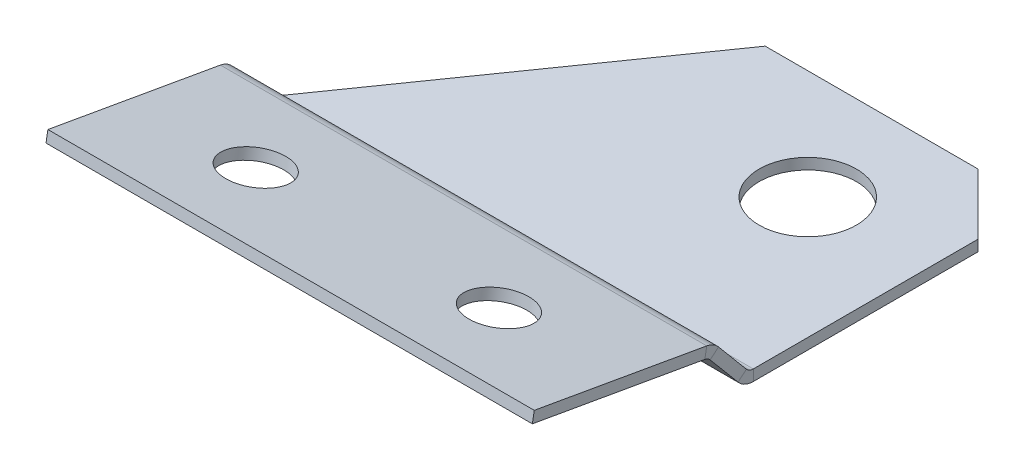
ISO-10303-21;
HEADER;
FILE_DESCRIPTION(('STEP AP214'),'2;1');
FILE_NAME('part.step','',(''),(''),'','','');
FILE_SCHEMA(('AUTOMOTIVE_DESIGN { 1 0 10303 214 1 1 1 1 }'));
ENDSEC;
DATA;
#1=APPLICATION_CONTEXT('core data for automotive mechanical design processes');
#2=APPLICATION_PROTOCOL_DEFINITION('international standard','automotive_design',2000,#1);
#3=PRODUCT_CONTEXT('',#1,'mechanical');
#4=PRODUCT('Part','Part','',(#3));
#5=PRODUCT_RELATED_PRODUCT_CATEGORY('part','',(#4));
#6=PRODUCT_DEFINITION_FORMATION('','',#4);
#7=PRODUCT_DEFINITION_CONTEXT('part definition',#1,'design');
#8=PRODUCT_DEFINITION('design','',#6,#7);
#9=PRODUCT_DEFINITION_SHAPE('','',#8);
#10=(LENGTH_UNIT() NAMED_UNIT(*) SI_UNIT(.MILLI.,.METRE.));
#11=(NAMED_UNIT(*) PLANE_ANGLE_UNIT() SI_UNIT($,.RADIAN.));
#12=(NAMED_UNIT(*) SI_UNIT($,.STERADIAN.) SOLID_ANGLE_UNIT());
#13=UNCERTAINTY_MEASURE_WITH_UNIT(LENGTH_MEASURE(1.E-05),#10,'distance_accuracy_value','');
#14=(GEOMETRIC_REPRESENTATION_CONTEXT(3) GLOBAL_UNCERTAINTY_ASSIGNED_CONTEXT((#13)) GLOBAL_UNIT_ASSIGNED_CONTEXT((#10,
#11,#12)) REPRESENTATION_CONTEXT('',''));
#15=CARTESIAN_POINT('',(0.,0.,0.));
#16=DIRECTION('',(0.,0.,1.));
#17=DIRECTION('',(1.,0.,0.));
#18=AXIS2_PLACEMENT_3D('',#15,#16,#17);
#19=CARTESIAN_POINT('',(-7.56166635581271,4.19626665871385,33.5211914025943));
#20=DIRECTION('',(-1.,0.,0.));
#21=DIRECTION('',(0.,0.,1.));
#22=AXIS2_PLACEMENT_3D('',#19,#20,#21);
#23=PLANE('',#22);
#24=DIRECTION('',(0.,0.766044443118975,0.642787609686544));
#25=VECTOR('',#24,1.);
#26=CARTESIAN_POINT('',(-7.56166635581271,4.19626665871385,33.5211914025943));
#27=LINE('',#26,#25);
#28=CARTESIAN_POINT('',(-7.56166635581271,0.184613797987,30.1550149667471));
#29=VERTEX_POINT('',#28);
#30=CARTESIAN_POINT('',(-7.56166635581271,2.91831154664444,32.4488597393957));
#31=VERTEX_POINT('',#30);
#32=EDGE_CURVE('E254',#29,#31,#27,.T.);
#33=ORIENTED_EDGE('',*,*,#32,.T.);
#34=DIRECTION('',(0.,0.642787609686544,-0.766044443118974));
#35=VECTOR('',#34,1.);
#36=CARTESIAN_POINT('',(-7.56166635581271,2.91831154664444,32.4488597393957));
#37=LINE('',#36,#35);
#38=CARTESIAN_POINT('',(-7.56166635581271,3.49682039536233,31.7594197405887));
#39=VERTEX_POINT('',#38);
#40=EDGE_CURVE('E241',#31,#39,#37,.T.);
#41=ORIENTED_EDGE('',*,*,#40,.T.);
#42=DIRECTION('',(0.,-0.766044443118975,-0.642787609686544));
#43=VECTOR('',#42,1.);
#44=CARTESIAN_POINT('',(-7.56166635581271,-14.7721682915287,16.4299180714363));
#45=LINE('',#44,#43);
#46=CARTESIAN_POINT('',(-7.56166635581271,0.76312264670489,29.46557496794));
#47=VERTEX_POINT('',#46);
#48=EDGE_CURVE('E259',#47,#39,#45,.F.);
#49=ORIENTED_EDGE('',*,*,#48,.F.);
#50=DIRECTION('',(0.,-0.642787609686544,0.766044443118974));
#51=VECTOR('',#50,1.);
#52=CARTESIAN_POINT('',(-7.56166635581271,0.184613797987001,30.1550149667471));
#53=LINE('',#52,#51);
#54=EDGE_CURVE('E247',#47,#29,#53,.T.);
#55=ORIENTED_EDGE('',*,*,#54,.T.);
#56=EDGE_LOOP('',(#33,#41,#49,#55));
#57=FACE_BOUND('',#56,.T.);
#58=ADVANCED_FACE('F81',(#57),#23,.T.);
#59=CARTESIAN_POINT('',(0.,-15.3506771402466,17.1193580702434));
#60=DIRECTION('',(0.,-0.642787609686544,0.766044443118975));
#61=DIRECTION('',(0.,-0.766044443118975,-0.642787609686544));
#62=AXIS2_PLACEMENT_3D('',#59,#60,#61);
#63=PLANE('',#62);
#64=DIRECTION('',(0.,-0.766044443118975,-0.642787609686544));
#65=VECTOR('',#64,1.);
#66=CARTESIAN_POINT('',(32.4383336441873,-0.0785088487178904,29.9342288509426));
#67=LINE('',#66,#65);
#68=CARTESIAN_POINT('',(32.4383336441873,2.91831154664445,32.4488597393957));
#69=VERTEX_POINT('',#68);
#70=CARTESIAN_POINT('',(32.4383336441873,0.184613797987,30.1550149667471));
#71=VERTEX_POINT('',#70);
#72=EDGE_CURVE('E249',#69,#71,#67,.T.);
#73=ORIENTED_EDGE('',*,*,#72,.F.);
#74=DIRECTION('',(-1.,0.,0.));
#75=VECTOR('',#74,1.);
#76=CARTESIAN_POINT('',(-7.56166635581271,2.91831154664444,32.4488597393957));
#77=LINE('',#76,#75);
#78=EDGE_CURVE('E107',#31,#69,#77,.F.);
#79=ORIENTED_EDGE('',*,*,#78,.F.);
#80=ORIENTED_EDGE('',*,*,#32,.F.);
#81=DIRECTION('',(1.,0.,0.));
#82=VECTOR('',#81,1.);
#83=CARTESIAN_POINT('',(0.,0.184613797986996,30.1550149667471));
#84=LINE('',#83,#82);
#85=EDGE_CURVE('E256',#29,#71,#84,.T.);
#86=ORIENTED_EDGE('',*,*,#85,.T.);
#87=EDGE_LOOP('',(#73,#79,#80,#86));
#88=FACE_BOUND('',#87,.T.);
#89=ADVANCED_FACE('F321',(#88),#63,.T.);
#90=CARTESIAN_POINT('',(0.,-14.7721682915287,16.4299180714363));
#91=DIRECTION('',(0.,-0.642787609686544,0.766044443118975));
#92=DIRECTION('',(0.,-0.766044443118975,-0.642787609686544));
#93=AXIS2_PLACEMENT_3D('',#90,#91,#92);
#94=PLANE('',#93);
#95=DIRECTION('',(-1.,0.,0.));
#96=VECTOR('',#95,1.);
#97=CARTESIAN_POINT('',(-7.56166635581271,3.49682039536233,31.7594197405887));
#98=LINE('',#97,#96);
#99=CARTESIAN_POINT('',(32.4383336441873,3.49682039536233,31.7594197405887));
#100=VERTEX_POINT('',#99);
#101=EDGE_CURVE('E188',#39,#100,#98,.F.);
#102=ORIENTED_EDGE('',*,*,#101,.T.);
#103=DIRECTION('',(0.,0.766044443118975,0.642787609686544));
#104=VECTOR('',#103,1.);
#105=CARTESIAN_POINT('',(32.4383336441873,-14.7721682915287,16.4299180714363));
#106=LINE('',#105,#104);
#107=CARTESIAN_POINT('',(32.4383336441873,0.76312264670489,29.46557496794));
#108=VERTEX_POINT('',#107);
#109=EDGE_CURVE('E253',#100,#108,#106,.F.);
#110=ORIENTED_EDGE('',*,*,#109,.T.);
#111=DIRECTION('',(-1.,0.,0.));
#112=VECTOR('',#111,1.);
#113=CARTESIAN_POINT('',(-7.56166635581271,0.763122646704892,29.46557496794));
#114=LINE('',#113,#112);
#115=EDGE_CURVE('E268',#47,#108,#114,.F.);
#116=ORIENTED_EDGE('',*,*,#115,.F.);
#117=ORIENTED_EDGE('',*,*,#48,.T.);
#118=EDGE_LOOP('',(#102,#110,#116,#117));
#119=FACE_BOUND('',#118,.T.);
#120=ADVANCED_FACE('F330',(#119),#94,.F.);
#121=CARTESIAN_POINT('',(32.4383336441873,0.5,0.));
#122=DIRECTION('',(-1.,0.,0.));
#123=DIRECTION('',(0.,0.,1.));
#124=AXIS2_PLACEMENT_3D('',#121,#122,#123);
#125=PLANE('',#124);
#126=DIRECTION('',(0.,0.,1.));
#127=VECTOR('',#126,1.);
#128=CARTESIAN_POINT('',(32.4383336441873,0.5,0.));
#129=LINE('',#128,#127);
#130=CARTESIAN_POINT('',(32.4383336441873,0.5,10.4196554125346));
#131=VERTEX_POINT('',#130);
#132=CARTESIAN_POINT('',(32.4383336441873,0.5,28.9013066311386));
#133=VERTEX_POINT('',#132);
#134=EDGE_CURVE('E379',#131,#133,#129,.T.);
#135=ORIENTED_EDGE('',*,*,#134,.T.);
#136=DIRECTION('',(0.,-1.,0.));
#137=VECTOR('',#136,1.);
#138=CARTESIAN_POINT('',(32.4383336441873,0.499999999999996,28.9013066311386));
#139=LINE('',#138,#137);
#140=CARTESIAN_POINT('',(32.4383336441873,-0.400000000000005,28.9013066311386));
#141=VERTEX_POINT('',#140);
#142=EDGE_CURVE('E282',#133,#141,#139,.T.);
#143=ORIENTED_EDGE('',*,*,#142,.T.);
#144=DIRECTION('',(0.,0.,1.));
#145=VECTOR('',#144,1.);
#146=CARTESIAN_POINT('',(32.4383336441873,-0.4,0.));
#147=LINE('',#146,#145);
#148=CARTESIAN_POINT('',(32.4383336441873,-0.4,10.4196554125346));
#149=VERTEX_POINT('',#148);
#150=EDGE_CURVE('E366',#149,#141,#147,.T.);
#151=ORIENTED_EDGE('',*,*,#150,.F.);
#152=DIRECTION('',(0.,1.,0.));
#153=VECTOR('',#152,1.);
#154=CARTESIAN_POINT('',(32.4383336441873,0.5,10.4196554125346));
#155=LINE('',#154,#153);
#156=EDGE_CURVE('E13',#149,#131,#155,.T.);
#157=ORIENTED_EDGE('',*,*,#156,.T.);
#158=EDGE_LOOP('',(#135,#143,#151,#157));
#159=FACE_BOUND('',#158,.T.);
#160=ADVANCED_FACE('F420',(#159),#125,.F.);
#161=CARTESIAN_POINT('',(9.21616941809498,0.5,6.45131859266648));
#162=DIRECTION('',(-0.81923192051904,0.,-0.573462344363328));
#163=DIRECTION('',(-0.573462344363328,0.,0.81923192051904));
#164=AXIS2_PLACEMENT_3D('',#161,#162,#163);
#165=PLANE('',#164);
#166=DIRECTION('',(-0.573462344363328,0.,0.81923192051904));
#167=VECTOR('',#166,1.);
#168=CARTESIAN_POINT('',(9.21616941809498,-0.4,6.45131859266648));
#169=LINE('',#168,#167);
#170=CARTESIAN_POINT('',(9.93833364418729,-0.4,5.41965541253461));
#171=VERTEX_POINT('',#170);
#172=CARTESIAN_POINT('',(-6.49882220883548,-0.4,28.9013066311386));
#173=VERTEX_POINT('',#172);
#174=EDGE_CURVE('E361',#171,#173,#169,.T.);
#175=ORIENTED_EDGE('',*,*,#174,.T.);
#176=DIRECTION('',(0.,-1.,0.));
#177=VECTOR('',#176,1.);
#178=CARTESIAN_POINT('',(-6.49882220883548,0.499999999999996,28.9013066311386));
#179=LINE('',#178,#177);
#180=CARTESIAN_POINT('',(-6.49882220883548,0.5,28.9013066311386));
#181=VERTEX_POINT('',#180);
#182=EDGE_CURVE('E281',#181,#173,#179,.T.);
#183=ORIENTED_EDGE('',*,*,#182,.F.);
#184=DIRECTION('',(-0.573462344363328,0.,0.81923192051904));
#185=VECTOR('',#184,1.);
#186=CARTESIAN_POINT('',(9.21616941809498,0.5,6.45131859266648));
#187=LINE('',#186,#185);
#188=CARTESIAN_POINT('',(9.93833364418729,0.5,5.41965541253461));
#189=VERTEX_POINT('',#188);
#190=EDGE_CURVE('E384',#189,#181,#187,.T.);
#191=ORIENTED_EDGE('',*,*,#190,.F.);
#192=DIRECTION('',(0.,1.,0.));
#193=VECTOR('',#192,1.);
#194=CARTESIAN_POINT('',(9.93833364418729,0.5,5.41965541253461));
#195=LINE('',#194,#193);
#196=EDGE_CURVE('E360',#171,#189,#195,.T.);
#197=ORIENTED_EDGE('',*,*,#196,.F.);
#198=EDGE_LOOP('',(#175,#183,#191,#197));
#199=FACE_BOUND('',#198,.T.);
#200=ADVANCED_FACE('F89',(#199),#165,.T.);
#201=CARTESIAN_POINT('',(0.,0.5,0.));
#202=DIRECTION('',(0.,1.,0.));
#203=DIRECTION('',(0.,0.,1.));
#204=AXIS2_PLACEMENT_3D('',#201,#202,#203);
#205=PLANE('',#204);
#206=CARTESIAN_POINT('',(22.4383336441873,0.5,14.4196554125346));
#207=DIRECTION('',(0.,1.,0.));
#208=DIRECTION('',(0.,0.,1.));
#209=AXIS2_PLACEMENT_3D('',#206,#207,#208);
#210=CIRCLE('',#209,4.);
#211=CARTESIAN_POINT('',(22.4383336441873,0.5,18.4196554125346));
#212=VERTEX_POINT('',#211);
#213=EDGE_CURVE('E373',#212,#212,#210,.T.);
#214=ORIENTED_EDGE('',*,*,#213,.F.);
#215=EDGE_LOOP('',(#214));
#216=FACE_BOUND('',#215,.T.);
#217=ORIENTED_EDGE('',*,*,#190,.T.);
#218=DIRECTION('',(1.,0.,0.));
#219=VECTOR('',#218,1.);
#220=CARTESIAN_POINT('',(32.4383336441873,0.499999999999996,28.9013066311386));
#221=LINE('',#220,#219);
#222=EDGE_CURVE('E277',#133,#181,#221,.F.);
#223=ORIENTED_EDGE('',*,*,#222,.F.);
#224=ORIENTED_EDGE('',*,*,#134,.F.);
#225=DIRECTION('',(0.707106781186548,0.,0.707106781186548));
#226=VECTOR('',#225,1.);
#227=CARTESIAN_POINT('',(11.0093391158263,0.5,-11.0093391158263));
#228=LINE('',#227,#226);
#229=CARTESIAN_POINT('',(27.4383336441873,0.5,5.41965541253461));
#230=VERTEX_POINT('',#229);
#231=EDGE_CURVE('E359',#230,#131,#228,.T.);
#232=ORIENTED_EDGE('',*,*,#231,.F.);
#233=DIRECTION('',(1.,0.,0.));
#234=VECTOR('',#233,1.);
#235=CARTESIAN_POINT('',(0.,0.5,5.41965541253461));
#236=LINE('',#235,#234);
#237=EDGE_CURVE('E388',#189,#230,#236,.T.);
#238=ORIENTED_EDGE('',*,*,#237,.F.);
#239=EDGE_LOOP('',(#217,#223,#224,#232,#238));
#240=FACE_BOUND('',#239,.T.);
#241=ADVANCED_FACE('F393',(#216,#240),#205,.T.);
#242=CARTESIAN_POINT('',(0.,-0.4,0.));
#243=DIRECTION('',(0.,1.,0.));
#244=DIRECTION('',(0.,0.,1.));
#245=AXIS2_PLACEMENT_3D('',#242,#243,#244);
#246=PLANE('',#245);
#247=CARTESIAN_POINT('',(22.4383336441873,-0.4,14.4196554125346));
#248=DIRECTION('',(0.,1.,0.));
#249=DIRECTION('',(0.,0.,1.));
#250=AXIS2_PLACEMENT_3D('',#247,#248,#249);
#251=CIRCLE('',#250,4.);
#252=CARTESIAN_POINT('',(22.4383336441873,-0.4,18.4196554125346));
#253=VERTEX_POINT('',#252);
#254=EDGE_CURVE('E288',#253,#253,#251,.T.);
#255=ORIENTED_EDGE('',*,*,#254,.T.);
#256=EDGE_LOOP('',(#255));
#257=FACE_BOUND('',#256,.T.);
#258=DIRECTION('',(1.,0.,0.));
#259=VECTOR('',#258,1.);
#260=CARTESIAN_POINT('',(32.4383336441873,-0.400000000000005,28.9013066311386));
#261=LINE('',#260,#259);
#262=EDGE_CURVE('E274',#141,#173,#261,.F.);
#263=ORIENTED_EDGE('',*,*,#262,.T.);
#264=ORIENTED_EDGE('',*,*,#174,.F.);
#265=DIRECTION('',(1.,0.,0.));
#266=VECTOR('',#265,1.);
#267=CARTESIAN_POINT('',(0.,-0.4,5.41965541253461));
#268=LINE('',#267,#266);
#269=CARTESIAN_POINT('',(27.4383336441873,-0.4,5.41965541253461));
#270=VERTEX_POINT('',#269);
#271=EDGE_CURVE('E370',#171,#270,#268,.T.);
#272=ORIENTED_EDGE('',*,*,#271,.T.);
#273=DIRECTION('',(0.707106781186548,0.,0.707106781186548));
#274=VECTOR('',#273,1.);
#275=CARTESIAN_POINT('',(11.0093391158263,-0.4,-11.0093391158263));
#276=LINE('',#275,#274);
#277=EDGE_CURVE('E369',#270,#149,#276,.T.);
#278=ORIENTED_EDGE('',*,*,#277,.T.);
#279=ORIENTED_EDGE('',*,*,#150,.T.);
#280=EDGE_LOOP('',(#263,#264,#272,#278,#279));
#281=FACE_BOUND('',#280,.T.);
#282=ADVANCED_FACE('F400',(#257,#281),#246,.F.);
#283=CARTESIAN_POINT('',(11.0093391158263,0.5,-11.0093391158263));
#284=DIRECTION('',(-0.707106781186548,0.,0.707106781186548));
#285=DIRECTION('',(0.707106781186548,0.,0.707106781186548));
#286=AXIS2_PLACEMENT_3D('',#283,#284,#285);
#287=PLANE('',#286);
#288=ORIENTED_EDGE('',*,*,#156,.F.);
#289=ORIENTED_EDGE('',*,*,#277,.F.);
#290=DIRECTION('',(0.,1.,0.));
#291=VECTOR('',#290,1.);
#292=CARTESIAN_POINT('',(27.4383336441873,0.5,5.41965541253461));
#293=LINE('',#292,#291);
#294=EDGE_CURVE('E92',#270,#230,#293,.T.);
#295=ORIENTED_EDGE('',*,*,#294,.T.);
#296=ORIENTED_EDGE('',*,*,#231,.T.);
#297=EDGE_LOOP('',(#288,#289,#295,#296));
#298=FACE_BOUND('',#297,.T.);
#299=ADVANCED_FACE('F421',(#298),#287,.F.);
#300=CARTESIAN_POINT('',(0.,0.5,5.41965541253461));
#301=DIRECTION('',(0.,0.,1.));
#302=DIRECTION('',(1.,0.,0.));
#303=AXIS2_PLACEMENT_3D('',#300,#301,#302);
#304=PLANE('',#303);
#305=ORIENTED_EDGE('',*,*,#294,.F.);
#306=ORIENTED_EDGE('',*,*,#271,.F.);
#307=ORIENTED_EDGE('',*,*,#196,.T.);
#308=ORIENTED_EDGE('',*,*,#237,.T.);
#309=EDGE_LOOP('',(#305,#306,#307,#308));
#310=FACE_BOUND('',#309,.T.);
#311=ADVANCED_FACE('F424',(#310),#304,.F.);
#312=CARTESIAN_POINT('',(22.4383336441873,0.5,14.4196554125346));
#313=DIRECTION('',(0.,1.,0.));
#314=DIRECTION('',(0.,0.,1.));
#315=AXIS2_PLACEMENT_3D('',#312,#313,#314);
#316=CYLINDRICAL_SURFACE('',#315,4.);
#317=ORIENTED_EDGE('',*,*,#213,.T.);
#318=EDGE_LOOP('',(#317));
#319=FACE_BOUND('',#318,.T.);
#320=ORIENTED_EDGE('',*,*,#254,.F.);
#321=EDGE_LOOP('',(#320));
#322=FACE_BOUND('',#321,.T.);
#323=ADVANCED_FACE('F391',(#319,#322),#316,.F.);
#324=CARTESIAN_POINT('',(-6.49882220883548,-0.409000000000004,28.9013066311386));
#325=CARTESIAN_POINT('',(-6.67599434589073,-0.409000000000004,29.1406918009645));
#326=CARTESIAN_POINT('',(-6.85310359116122,-0.355970740088898,29.3798489828527));
#327=CARTESIAN_POINT('',(-7.20738497348696,-0.153669448606135,29.8136855024655));
#328=CARTESIAN_POINT('',(-7.38449421875746,-0.00455096961041456,30.0080355456284));
#329=CARTESIAN_POINT('',(-7.56166635581271,0.178828709499822,30.1619093667352));
#330=CARTESIAN_POINT('',(-6.49882220883548,-0.400000000000004,28.9013066311386));
#331=CARTESIAN_POINT('',(-6.67599416335543,-0.400000000000004,29.1393824626054));
#332=CARTESIAN_POINT('',(-6.85310359116122,-0.347260763994585,29.377231772616));
#333=CARTESIAN_POINT('',(-7.20738497348696,-0.146065884533788,29.8086955839908));
#334=CARTESIAN_POINT('',(-7.38449440129276,0.00223713025094104,30.0019827721144));
#335=CARTESIAN_POINT('',(-7.56166635581271,0.184613797987001,30.1550149667471));
#336=CARTESIAN_POINT('',(-6.49882220883548,0.499999999999996,28.9013066311386));
#337=CARTESIAN_POINT('',(-6.67597590982505,0.499999999999996,29.008448626692));
#338=CARTESIAN_POINT('',(-6.85310359116122,0.523736845436628,29.1155107489513));
#339=CARTESIAN_POINT('',(-7.20738497348696,0.614290522700971,29.3097037365223));
#340=CARTESIAN_POINT('',(-7.38451265482314,0.681047116386501,29.3967054207212));
#341=CARTESIAN_POINT('',(-7.56166635581271,0.76312264670489,29.46557496794));
#342=CARTESIAN_POINT('',(-6.49882220883548,0.509089999999996,28.9013066311386));
#343=CARTESIAN_POINT('',(-6.67597572546439,0.509089999999996,29.0071261949493));
#344=CARTESIAN_POINT('',(-6.85310359116122,0.532533921291883,29.1128673666123));
#345=CARTESIAN_POINT('',(-7.20738497348696,0.621970122414042,29.3046639188628));
#346=CARTESIAN_POINT('',(-7.3845128391838,0.68790309724647,29.3905921194721));
#347=CARTESIAN_POINT('',(-7.56166635581271,0.76896558607694,29.4586116239521));
#348=B_SPLINE_SURFACE_WITH_KNOTS('',1,3,((#324,#325,#326,#327,#328,#329),(#330,#331,#332,#333,
#334,#335),(#336,#337,#338,#339,#340,#341),(#342,#343,#344,#345,#346,#347)),.UNSPECIFIED.,.F.,
.F.,.F.,(2,1,1,2),(4,2,4),(-0.01,0.,1.,1.0101),(0.,0.5,1.),.UNSPECIFIED.);
#349=CARTESIAN_POINT('',(-6.49882220883548,0.499999999999996,28.9013066311386));
#350=CARTESIAN_POINT('',(-6.5515147636366,0.499987366324268,28.9331716583041));
#351=CARTESIAN_POINT('',(-6.60420460339763,0.502067142913907,28.9650370339194));
#352=CARTESIAN_POINT('',(-6.7095672477327,0.510321127633015,29.0282259966509));
#353=CARTESIAN_POINT('',(-6.76224005270163,0.516494114720724,29.0595497424817));
#354=CARTESIAN_POINT('',(-6.86759293380989,0.532844927931029,29.1211352250849));
#355=CARTESIAN_POINT('',(-6.92027301018619,0.543023095625512,29.1513968710389));
#356=CARTESIAN_POINT('',(-7.02563555769857,0.567206544951451,29.2103496843492));
#357=CARTESIAN_POINT('',(-7.07831802828386,0.581212314286158,29.2390406510139));
#358=CARTESIAN_POINT('',(-7.20275252228463,0.618547641012969,29.3043828793143));
#359=CARTESIAN_POINT('',(-7.27451206466591,0.643417380651416,29.340161405879));
#360=CARTESIAN_POINT('',(-7.38215545184342,0.68514686995654,29.3901338881046));
#361=CARTESIAN_POINT('',(-7.41805717847375,0.699803541050182,29.4061833741658));
#362=CARTESIAN_POINT('',(-7.48985920751327,0.730473964765427,29.4369254004144));
#363=CARTESIAN_POINT('',(-7.52575950989105,0.746487642100447,29.4516180157865));
#364=CARTESIAN_POINT('',(-7.56166635581271,0.76312264670489,29.46557496794));
#365=B_SPLINE_CURVE_WITH_KNOTS('',3,(#349,#350,#351,#352,#353,#354,#355,#356,#357,#358,#359,
#360,#361,#362,#363,#364),.UNSPECIFIED.,.F.,.F.,(4,2,2,2,2,2,2,4),(0.,0.184696314357836,
0.369337556904419,0.553994549534938,0.738675081667851,0.990131805299582,1.11599990262725,
1.24186102137066),.UNSPECIFIED.);
#366=EDGE_CURVE('E273',#181,#47,#365,.T.);
#367=CARTESIAN_POINT('',(-6.49882220883548,-0.400000000000004,28.9013066311386));
#368=CARTESIAN_POINT('',(-6.54160660347905,-0.40001203454415,28.9587939693427));
#369=CARTESIAN_POINT('',(-6.58438930905709,-0.396971564152638,29.0162804262751));
#370=CARTESIAN_POINT('',(-6.66996656829968,-0.384869570642051,29.1306371263556));
#371=CARTESIAN_POINT('',(-6.71276112124318,-0.375806071273359,29.1875071610192));
#372=CARTESIAN_POINT('',(-6.79817634138095,-0.351790685857574,29.2997508207635));
#373=CARTESIAN_POINT('',(-6.84079701266502,-0.336862734502081,29.3551295627252));
#374=CARTESIAN_POINT('',(-6.92602272721566,-0.301295967616742,29.4639901027199));
#375=CARTESIAN_POINT('',(-6.96862776898845,-0.280659698502557,29.5174727346125));
#376=CARTESIAN_POINT('',(-7.05635786139815,-0.232514405014484,29.6250731073271));
#377=CARTESIAN_POINT('',(-7.1014830548518,-0.204671317458185,29.6790416272596));
#378=CARTESIAN_POINT('',(-7.19170963581545,-0.143184762814139,29.7835357405012));
#379=CARTESIAN_POINT('',(-7.23681102511457,-0.10954383453105,29.8340628273177));
#380=CARTESIAN_POINT('',(-7.32851790904156,-0.0356514360091606,29.9326910202602));
#381=CARTESIAN_POINT('',(-7.37512344501756,0.00478295692197111,29.9806551853378));
#382=CARTESIAN_POINT('',(-7.46837409896036,0.0909013280280136,30.0716819025853));
#383=CARTESIAN_POINT('',(-7.51501921903862,0.136589439042174,30.1147405420821));
#384=CARTESIAN_POINT('',(-7.56166635581271,0.184613797987001,30.1550149667471));
#385=B_SPLINE_CURVE_WITH_KNOTS('',3,(#367,#368,#369,#370,#371,#372,#373,#374,#375,#376,#377,
#378,#379,#380,#381,#382,#383,#384),.UNSPECIFIED.,.F.,.F.,(4,2,2,2,2,2,2,2,4),(0.,
0.214916121277141,0.429902794721954,0.644021005719627,0.858043854625659,1.0847136154163,
1.31128437126926,1.54540489758131,1.7797108713141),.UNSPECIFIED.);
#386=EDGE_CURVE('E284',#173,#29,#385,.T.);
#387=ORIENTED_EDGE('',*,*,#54,.F.);
#388=ORIENTED_EDGE('',*,*,#366,.F.);
#389=ORIENTED_EDGE('',*,*,#182,.T.);
#390=ORIENTED_EDGE('',*,*,#386,.T.);
#391=EDGE_LOOP('',(#387,#388,#389,#390));
#392=FACE_BOUND('',#391,.T.);
#393=ADVANCED_FACE('F303',(#392),#348,.F.);
#394=CARTESIAN_POINT('',(32.4383336441873,1.2366,28.9013066311386));
#395=DIRECTION('',(-1.,0.,0.));
#396=DIRECTION('',(0.,0.,1.));
#397=AXIS2_PLACEMENT_3D('',#394,#395,#396);
#398=PLANE('',#397);
#399=CARTESIAN_POINT('',(32.4383336441873,1.2366,28.9013066311386));
#400=DIRECTION('',(1.,0.,0.));
#401=DIRECTION('',(0.,0.,-1.));
#402=AXIS2_PLACEMENT_3D('',#399,#400,#401);
#403=CIRCLE('',#402,0.736600000000005);
#404=EDGE_CURVE('E255',#108,#133,#403,.T.);
#405=ORIENTED_EDGE('',*,*,#404,.F.);
#406=DIRECTION('',(0.,-0.642787609686544,0.766044443118974));
#407=VECTOR('',#406,1.);
#408=CARTESIAN_POINT('',(32.4383336441873,0.763122646704892,29.46557496794));
#409=LINE('',#408,#407);
#410=EDGE_CURVE('E264',#108,#71,#409,.T.);
#411=ORIENTED_EDGE('',*,*,#410,.T.);
#412=CARTESIAN_POINT('',(32.4383336441873,1.2366,28.9013066311386));
#413=DIRECTION('',(1.,0.,0.));
#414=DIRECTION('',(0.,0.,-1.));
#415=AXIS2_PLACEMENT_3D('',#412,#413,#414);
#416=CIRCLE('',#415,1.6366);
#417=EDGE_CURVE('E272',#71,#141,#416,.T.);
#418=ORIENTED_EDGE('',*,*,#417,.T.);
#419=ORIENTED_EDGE('',*,*,#142,.F.);
#420=EDGE_LOOP('',(#405,#411,#418,#419));
#421=FACE_BOUND('',#420,.T.);
#422=ADVANCED_FACE('F312',(#421),#398,.F.);
#423=CARTESIAN_POINT('',(32.4383336441873,1.2366,28.9013066311386));
#424=DIRECTION('',(1.,0.,0.));
#425=DIRECTION('',(0.,-0.642787609686544,0.766044443118975));
#426=AXIS2_PLACEMENT_3D('',#423,#424,#425);
#427=CYLINDRICAL_SURFACE('',#426,1.6366);
#428=ORIENTED_EDGE('',*,*,#262,.F.);
#429=ORIENTED_EDGE('',*,*,#417,.F.);
#430=ORIENTED_EDGE('',*,*,#85,.F.);
#431=ORIENTED_EDGE('',*,*,#386,.F.);
#432=EDGE_LOOP('',(#428,#429,#430,#431));
#433=FACE_BOUND('',#432,.T.);
#434=ADVANCED_FACE('F308',(#433),#427,.T.);
#435=CARTESIAN_POINT('',(32.4383336441873,1.2366,28.9013066311386));
#436=DIRECTION('',(1.,0.,0.));
#437=DIRECTION('',(0.,-0.642787609686544,0.766044443118975));
#438=AXIS2_PLACEMENT_3D('',#435,#436,#437);
#439=CYLINDRICAL_SURFACE('',#438,0.736600000000005);
#440=ORIENTED_EDGE('',*,*,#222,.T.);
#441=ORIENTED_EDGE('',*,*,#366,.T.);
#442=ORIENTED_EDGE('',*,*,#115,.T.);
#443=ORIENTED_EDGE('',*,*,#404,.T.);
#444=EDGE_LOOP('',(#440,#441,#442,#443));
#445=FACE_BOUND('',#444,.T.);
#446=ADVANCED_FACE('F315',(#445),#439,.F.);
#447=CARTESIAN_POINT('',(32.4383336441873,-0.0785088487178904,29.9342288509426));
#448=DIRECTION('',(1.,0.,0.));
#449=DIRECTION('',(0.,0.,-1.));
#450=AXIS2_PLACEMENT_3D('',#447,#448,#449);
#451=PLANE('',#450);
#452=DIRECTION('',(0.,0.642787609686544,-0.766044443118974));
#453=VECTOR('',#452,1.);
#454=CARTESIAN_POINT('',(32.4383336441873,2.91831154664444,32.4488597393957));
#455=LINE('',#454,#453);
#456=EDGE_CURVE('E105',#69,#100,#455,.T.);
#457=ORIENTED_EDGE('',*,*,#456,.F.);
#458=ORIENTED_EDGE('',*,*,#72,.T.);
#459=ORIENTED_EDGE('',*,*,#410,.F.);
#460=ORIENTED_EDGE('',*,*,#109,.F.);
#461=EDGE_LOOP('',(#457,#458,#459,#460));
#462=FACE_BOUND('',#461,.T.);
#463=ADVANCED_FACE('F319',(#462),#451,.T.);
#464=CARTESIAN_POINT('',(32.4383336441873,2.44483419334933,33.0131280761972));
#465=DIRECTION('',(1.,0.,0.));
#466=DIRECTION('',(0.,0.,-1.));
#467=AXIS2_PLACEMENT_3D('',#464,#465,#466);
#468=PLANE('',#467);
#469=DIRECTION('',(0.,0.984807753012208,-0.17364817766693));
#470=VECTOR('',#469,1.);
#471=CARTESIAN_POINT('',(32.4383336441873,4.05657056192911,32.7289354686275));
#472=LINE('',#471,#470);
#473=CARTESIAN_POINT('',(32.4383336441873,3.17024358421812,32.8852188285277));
#474=VERTEX_POINT('',#473);
#475=CARTESIAN_POINT('',(32.4383336441873,4.05657056192911,32.7289354686275));
#476=VERTEX_POINT('',#475);
#477=EDGE_CURVE('E232',#474,#476,#472,.T.);
#478=ORIENTED_EDGE('',*,*,#477,.F.);
#479=CARTESIAN_POINT('',(32.4383336441873,2.44483419334933,33.0131280761972));
#480=DIRECTION('',(-1.,0.,0.));
#481=DIRECTION('',(0.,0.,1.));
#482=AXIS2_PLACEMENT_3D('',#479,#480,#481);
#483=CIRCLE('',#482,0.736599999999996);
#484=EDGE_CURVE('E192',#69,#474,#483,.F.);
#485=ORIENTED_EDGE('',*,*,#484,.F.);
#486=ORIENTED_EDGE('',*,*,#456,.T.);
#487=CARTESIAN_POINT('',(32.4383336441873,2.44483419334933,33.0131280761972));
#488=DIRECTION('',(-1.,0.,0.));
#489=DIRECTION('',(0.,0.,1.));
#490=AXIS2_PLACEMENT_3D('',#487,#488,#489);
#491=CIRCLE('',#490,1.6366);
#492=EDGE_CURVE('E239',#100,#476,#491,.F.);
#493=ORIENTED_EDGE('',*,*,#492,.T.);
#494=EDGE_LOOP('',(#478,#485,#486,#493));
#495=FACE_BOUND('',#494,.T.);
#496=ADVANCED_FACE('F325',(#495),#468,.T.);
#497=CARTESIAN_POINT('',(-7.56166635581271,2.44483419334933,33.0131280761972));
#498=DIRECTION('',(1.,0.,0.));
#499=DIRECTION('',(0.,0.,-1.));
#500=AXIS2_PLACEMENT_3D('',#497,#498,#499);
#501=PLANE('',#500);
#502=CARTESIAN_POINT('',(-7.56166635581271,2.44483419334933,33.0131280761972));
#503=DIRECTION('',(-1.,0.,0.));
#504=DIRECTION('',(0.,0.,1.));
#505=AXIS2_PLACEMENT_3D('',#502,#503,#504);
#506=CIRCLE('',#505,0.736599999999996);
#507=CARTESIAN_POINT('',(-7.56166635581271,3.17024358421812,32.8852188285277));
#508=VERTEX_POINT('',#507);
#509=EDGE_CURVE('E200',#508,#31,#506,.T.);
#510=ORIENTED_EDGE('',*,*,#509,.F.);
#511=DIRECTION('',(0.,0.984807753012208,-0.17364817766693));
#512=VECTOR('',#511,1.);
#513=CARTESIAN_POINT('',(-7.56166635581271,3.17024358421812,32.8852188285277));
#514=LINE('',#513,#512);
#515=CARTESIAN_POINT('',(-7.56166635581271,4.05657056192911,32.7289354686275));
#516=VERTEX_POINT('',#515);
#517=EDGE_CURVE('E197',#508,#516,#514,.T.);
#518=ORIENTED_EDGE('',*,*,#517,.T.);
#519=CARTESIAN_POINT('',(-7.56166635581271,2.44483419334933,33.0131280761972));
#520=DIRECTION('',(-1.,0.,0.));
#521=DIRECTION('',(0.,0.,1.));
#522=AXIS2_PLACEMENT_3D('',#519,#520,#521);
#523=CIRCLE('',#522,1.6366);
#524=EDGE_CURVE('E182',#516,#39,#523,.T.);
#525=ORIENTED_EDGE('',*,*,#524,.T.);
#526=ORIENTED_EDGE('',*,*,#40,.F.);
#527=EDGE_LOOP('',(#510,#518,#525,#526));
#528=FACE_BOUND('',#527,.T.);
#529=ADVANCED_FACE('F199',(#528),#501,.F.);
#530=CARTESIAN_POINT('',(-7.56166635581271,2.44483419334933,33.0131280761972));
#531=DIRECTION('',(-1.,0.,0.));
#532=DIRECTION('',(0.,0.984807753012208,-0.17364817766693));
#533=AXIS2_PLACEMENT_3D('',#530,#531,#532);
#534=CYLINDRICAL_SURFACE('',#533,1.6366);
#535=ORIENTED_EDGE('',*,*,#101,.F.);
#536=ORIENTED_EDGE('',*,*,#524,.F.);
#537=DIRECTION('',(-1.,0.,0.));
#538=VECTOR('',#537,1.);
#539=CARTESIAN_POINT('',(0.,4.05657056192911,32.7289354686275));
#540=LINE('',#539,#538);
#541=EDGE_CURVE('E189',#476,#516,#540,.T.);
#542=ORIENTED_EDGE('',*,*,#541,.F.);
#543=ORIENTED_EDGE('',*,*,#492,.F.);
#544=EDGE_LOOP('',(#535,#536,#542,#543));
#545=FACE_BOUND('',#544,.T.);
#546=ADVANCED_FACE('F184',(#545),#534,.T.);
#547=CARTESIAN_POINT('',(-7.56166635581271,2.44483419334933,33.0131280761972));
#548=DIRECTION('',(-1.,0.,0.));
#549=DIRECTION('',(0.,0.984807753012208,-0.17364817766693));
#550=AXIS2_PLACEMENT_3D('',#547,#548,#549);
#551=CYLINDRICAL_SURFACE('',#550,0.736599999999996);
#552=ORIENTED_EDGE('',*,*,#78,.T.);
#553=ORIENTED_EDGE('',*,*,#484,.T.);
#554=DIRECTION('',(1.,0.,0.));
#555=VECTOR('',#554,1.);
#556=CARTESIAN_POINT('',(32.4383336441873,3.17024358421812,32.8852188285277));
#557=LINE('',#556,#555);
#558=EDGE_CURVE('E202',#474,#508,#557,.F.);
#559=ORIENTED_EDGE('',*,*,#558,.T.);
#560=ORIENTED_EDGE('',*,*,#509,.T.);
#561=EDGE_LOOP('',(#552,#553,#559,#560));
#562=FACE_BOUND('',#561,.T.);
#563=ADVANCED_FACE('F334',(#562),#551,.F.);
#564=CARTESIAN_POINT('',(-7.56166635581271,4.01001540309004,32.4649080426941));
#565=DIRECTION('',(-1.,0.,0.));
#566=DIRECTION('',(0.,0.,1.));
#567=AXIS2_PLACEMENT_3D('',#564,#565,#566);
#568=PLANE('',#567);
#569=DIRECTION('',(0.,-0.17364817766693,-0.984807753012208));
#570=VECTOR('',#569,1.);
#571=CARTESIAN_POINT('',(-7.56166635581271,4.01001540309004,32.4649080426941));
#572=LINE('',#571,#570);
#573=CARTESIAN_POINT('',(-7.56166635581271,6.5578555769792,46.9144277001633));
#574=VERTEX_POINT('',#573);
#575=EDGE_CURVE('E214',#574,#516,#572,.T.);
#576=ORIENTED_EDGE('',*,*,#575,.T.);
#577=ORIENTED_EDGE('',*,*,#517,.F.);
#578=DIRECTION('',(0.,0.17364817766693,0.984807753012208));
#579=VECTOR('',#578,1.);
#580=CARTESIAN_POINT('',(-7.56166635581271,-2.73530584093744,-0.606816261210827));
#581=LINE('',#580,#579);
#582=CARTESIAN_POINT('',(-7.56166635581271,5.67152859926821,47.0707110600635));
#583=VERTEX_POINT('',#582);
#584=EDGE_CURVE('E226',#583,#508,#581,.F.);
#585=ORIENTED_EDGE('',*,*,#584,.F.);
#586=DIRECTION('',(0.,-0.984807753012208,0.17364817766693));
#587=VECTOR('',#586,1.);
#588=CARTESIAN_POINT('',(-7.56166635581271,6.5578555769792,46.9144277001633));
#589=LINE('',#588,#587);
#590=EDGE_CURVE('E219',#574,#583,#589,.T.);
#591=ORIENTED_EDGE('',*,*,#590,.F.);
#592=EDGE_LOOP('',(#576,#577,#585,#591));
#593=FACE_BOUND('',#592,.T.);
#594=ADVANCED_FACE('F218',(#593),#568,.T.);
#595=CARTESIAN_POINT('',(32.4383336441873,6.5578555769792,46.9144277001633));
#596=DIRECTION('',(1.,0.,0.));
#597=DIRECTION('',(0.,0.,-1.));
#598=AXIS2_PLACEMENT_3D('',#595,#596,#597);
#599=PLANE('',#598);
#600=DIRECTION('',(0.,-0.17364817766693,-0.984807753012208));
#601=VECTOR('',#600,1.);
#602=CARTESIAN_POINT('',(32.4383336441873,-2.73530584093744,-0.606816261210813));
#603=LINE('',#602,#601);
#604=CARTESIAN_POINT('',(32.4383336441873,5.67152859926821,47.0707110600635));
#605=VERTEX_POINT('',#604);
#606=EDGE_CURVE('E215',#474,#605,#603,.F.);
#607=ORIENTED_EDGE('',*,*,#606,.F.);
#608=ORIENTED_EDGE('',*,*,#477,.T.);
#609=DIRECTION('',(0.,0.17364817766693,0.984807753012208));
#610=VECTOR('',#609,1.);
#611=CARTESIAN_POINT('',(32.4383336441873,6.5578555769792,46.9144277001633));
#612=LINE('',#611,#610);
#613=CARTESIAN_POINT('',(32.4383336441873,6.5578555769792,46.9144277001633));
#614=VERTEX_POINT('',#613);
#615=EDGE_CURVE('E212',#476,#614,#612,.T.);
#616=ORIENTED_EDGE('',*,*,#615,.T.);
#617=DIRECTION('',(0.,-0.984807753012208,0.17364817766693));
#618=VECTOR('',#617,1.);
#619=CARTESIAN_POINT('',(32.4383336441873,6.5578555769792,46.9144277001633));
#620=LINE('',#619,#618);
#621=EDGE_CURVE('E220',#614,#605,#620,.T.);
#622=ORIENTED_EDGE('',*,*,#621,.T.);
#623=EDGE_LOOP('',(#607,#608,#616,#622));
#624=FACE_BOUND('',#623,.T.);
#625=ADVANCED_FACE('F343',(#624),#599,.T.);
#626=CARTESIAN_POINT('',(0.,-1.84897886322645,-0.763099621111065));
#627=DIRECTION('',(0.,0.984807753012208,-0.17364817766693));
#628=DIRECTION('',(0.,0.17364817766693,0.984807753012208));
#629=AXIS2_PLACEMENT_3D('',#626,#627,#628);
#630=PLANE('',#629);
#631=CARTESIAN_POINT('',(2.43833364418729,5.30721306945416,39.8216815843954));
#632=DIRECTION('',(0.,0.984807753012208,-0.17364817766693));
#633=DIRECTION('',(0.,0.17364817766693,0.984807753012208));
#634=AXIS2_PLACEMENT_3D('',#631,#632,#633);
#635=CIRCLE('',#634,2.5);
#636=CARTESIAN_POINT('',(2.43833364418729,5.74133351362148,42.2837009669259));
#637=VERTEX_POINT('',#636);
#638=EDGE_CURVE('E238',#637,#637,#635,.T.);
#639=ORIENTED_EDGE('',*,*,#638,.F.);
#640=EDGE_LOOP('',(#639));
#641=FACE_BOUND('',#640,.T.);
#642=CARTESIAN_POINT('',(22.4383336441873,5.30721306945416,39.8216815843954));
#643=DIRECTION('',(0.,0.984807753012208,-0.17364817766693));
#644=DIRECTION('',(0.,0.17364817766693,0.984807753012208));
#645=AXIS2_PLACEMENT_3D('',#642,#643,#644);
#646=CIRCLE('',#645,2.5);
#647=CARTESIAN_POINT('',(22.4383336441873,5.74133351362148,42.2837009669259));
#648=VERTEX_POINT('',#647);
#649=EDGE_CURVE('E350',#648,#648,#646,.T.);
#650=ORIENTED_EDGE('',*,*,#649,.F.);
#651=EDGE_LOOP('',(#650));
#652=FACE_BOUND('',#651,.T.);
#653=ORIENTED_EDGE('',*,*,#615,.F.);
#654=ORIENTED_EDGE('',*,*,#541,.T.);
#655=ORIENTED_EDGE('',*,*,#575,.F.);
#656=DIRECTION('',(-1.,0.,0.));
#657=VECTOR('',#656,1.);
#658=CARTESIAN_POINT('',(-7.56166635581271,6.5578555769792,46.9144277001633));
#659=LINE('',#658,#657);
#660=EDGE_CURVE('E216',#614,#574,#659,.T.);
#661=ORIENTED_EDGE('',*,*,#660,.F.);
#662=EDGE_LOOP('',(#653,#654,#655,#661));
#663=FACE_BOUND('',#662,.T.);
#664=ADVANCED_FACE('F208',(#641,#652,#663),#630,.T.);
#665=CARTESIAN_POINT('',(0.,-2.73530584093744,-0.606816261210828));
#666=DIRECTION('',(0.,0.984807753012208,-0.17364817766693));
#667=DIRECTION('',(0.,0.17364817766693,0.984807753012208));
#668=AXIS2_PLACEMENT_3D('',#665,#666,#667);
#669=PLANE('',#668);
#670=CARTESIAN_POINT('',(2.43833364418729,4.42088609174317,39.9779649442956));
#671=DIRECTION('',(0.,0.984807753012208,-0.17364817766693));
#672=DIRECTION('',(0.,0.17364817766693,0.984807753012208));
#673=AXIS2_PLACEMENT_3D('',#670,#671,#672);
#674=CIRCLE('',#673,2.5);
#675=CARTESIAN_POINT('',(2.43833364418729,4.85500653591049,42.4399843268261));
#676=VERTEX_POINT('',#675);
#677=EDGE_CURVE('E90',#676,#676,#674,.T.);
#678=ORIENTED_EDGE('',*,*,#677,.T.);
#679=EDGE_LOOP('',(#678));
#680=FACE_BOUND('',#679,.T.);
#681=CARTESIAN_POINT('',(22.4383336441873,4.42088609174317,39.9779649442956));
#682=DIRECTION('',(0.,0.984807753012208,-0.17364817766693));
#683=DIRECTION('',(0.,0.17364817766693,0.984807753012208));
#684=AXIS2_PLACEMENT_3D('',#681,#682,#683);
#685=CIRCLE('',#684,2.5);
#686=CARTESIAN_POINT('',(22.4383336441873,4.85500653591049,42.4399843268261));
#687=VERTEX_POINT('',#686);
#688=EDGE_CURVE('E351',#687,#687,#685,.T.);
#689=ORIENTED_EDGE('',*,*,#688,.T.);
#690=EDGE_LOOP('',(#689));
#691=FACE_BOUND('',#690,.T.);
#692=ORIENTED_EDGE('',*,*,#558,.F.);
#693=ORIENTED_EDGE('',*,*,#606,.T.);
#694=DIRECTION('',(1.,0.,0.));
#695=VECTOR('',#694,1.);
#696=CARTESIAN_POINT('',(0.,5.67152859926821,47.0707110600635));
#697=LINE('',#696,#695);
#698=EDGE_CURVE('E229',#605,#583,#697,.F.);
#699=ORIENTED_EDGE('',*,*,#698,.T.);
#700=ORIENTED_EDGE('',*,*,#584,.T.);
#701=EDGE_LOOP('',(#692,#693,#699,#700));
#702=FACE_BOUND('',#701,.T.);
#703=ADVANCED_FACE('F339',(#680,#691,#702),#669,.F.);
#704=CARTESIAN_POINT('',(-7.56166635581271,6.5578555769792,46.9144277001633));
#705=DIRECTION('',(0.,0.17364817766693,0.984807753012208));
#706=DIRECTION('',(0.,-0.984807753012208,0.17364817766693));
#707=AXIS2_PLACEMENT_3D('',#704,#705,#706);
#708=PLANE('',#707);
#709=ORIENTED_EDGE('',*,*,#698,.F.);
#710=ORIENTED_EDGE('',*,*,#621,.F.);
#711=ORIENTED_EDGE('',*,*,#660,.T.);
#712=ORIENTED_EDGE('',*,*,#590,.T.);
#713=EDGE_LOOP('',(#709,#710,#711,#712));
#714=FACE_BOUND('',#713,.T.);
#715=ADVANCED_FACE('F341',(#714),#708,.T.);
#716=CARTESIAN_POINT('',(22.4383336441873,-1.46756351870241,41.0162574851594));
#717=DIRECTION('',(0.,0.984807753012208,-0.17364817766693));
#718=DIRECTION('',(0.,0.17364817766693,0.984807753012208));
#719=AXIS2_PLACEMENT_3D('',#716,#717,#718);
#720=CYLINDRICAL_SURFACE('',#719,2.5);
#721=ORIENTED_EDGE('',*,*,#649,.T.);
#722=EDGE_LOOP('',(#721));
#723=FACE_BOUND('',#722,.T.);
#724=ORIENTED_EDGE('',*,*,#688,.F.);
#725=EDGE_LOOP('',(#724));
#726=FACE_BOUND('',#725,.T.);
#727=ADVANCED_FACE('F607',(#723,#726),#720,.F.);
#728=CARTESIAN_POINT('',(2.43833364418729,-1.46756351870241,41.0162574851594));
#729=DIRECTION('',(0.,0.984807753012208,-0.17364817766693));
#730=DIRECTION('',(0.,0.17364817766693,0.984807753012208));
#731=AXIS2_PLACEMENT_3D('',#728,#729,#730);
#732=CYLINDRICAL_SURFACE('',#731,2.5);
#733=ORIENTED_EDGE('',*,*,#638,.T.);
#734=EDGE_LOOP('',(#733));
#735=FACE_BOUND('',#734,.T.);
#736=ORIENTED_EDGE('',*,*,#677,.F.);
#737=EDGE_LOOP('',(#736));
#738=FACE_BOUND('',#737,.T.);
#739=ADVANCED_FACE('F616',(#735,#738),#732,.F.);
#740=CLOSED_SHELL('',(#58,#89,#120,#160,#200,#241,#282,#299,#311,#323,#393,#422,#434,#446,#463,
#496,#529,#546,#563,#594,#625,#664,#703,#715,#727,#739));
#741=MANIFOLD_SOLID_BREP('B2',#740);
#742=ADVANCED_BREP_SHAPE_REPRESENTATION('',(#18,#741),#14);
#743=SHAPE_DEFINITION_REPRESENTATION(#9,#742);
ENDSEC;
END-ISO-10303-21;
